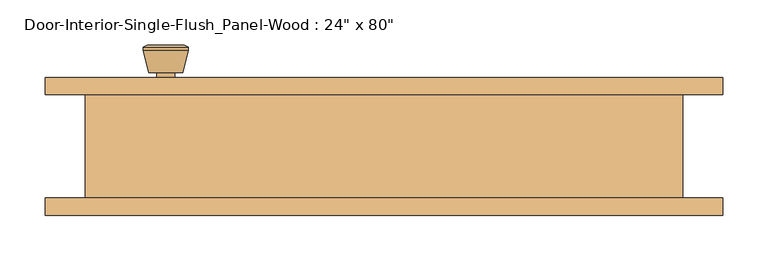
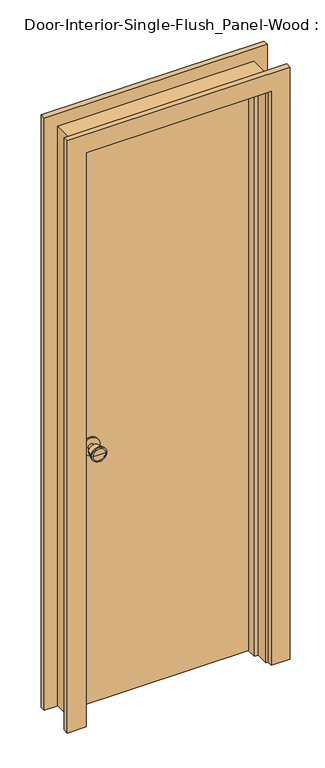
"""IFC4 building model written with IfcOpenShell, lengths in millimetres: door geometry."""

from ifc_helpers import new_model, si_unit, point, frame, frame_2d, origin, origin_with_axes, place, context, project, spatial, polyline, circle_curve, trimmed, segment, composite_curve, outline, extrude, faceted_brep, source, transform, mapped, element, save
from ifc_brep_helpers import plane_surface, cylinder_surface, revolved_surface, advanced_brep


def door_0e119d28(model_context):
    return source(origin(), model_context, "Body", "SolidModel", [
        advanced_brep(
        [(-241.3, 13.05, 914.4), (-231.3, 13.05, 914.4), (-251.3, 13.05, 914.4), (-220.8241324, -35.95, 914.4), (-241.3, -35.95, 914.4), (-261.7758676, -35.95, 914.4), (-216.3, -34.1221319, 914.4), (-266.3, -34.1221319, 914.4), (-216.3, -30.6584537, 914.4), (-266.3, -30.6584537, 914.4), (-222.663764, -5.95, 914.4), (-259.936236, -5.95, 914.4), (-231.3, -5.95, 914.4), (-251.3, -5.95, 914.4)],
        [
            (0, 1),
            (1, 2, circle_curve(frame((-241.3, 13.05, 914.4), z_axis=(0.0, 1.0, 0.0), x_axis=(-1.0, 0.0, 0.0)), 10.0)),
            (2, 0),
            (2, 1, circle_curve(frame((-241.3, 13.05, 914.4), z_axis=(0.0, 1.0, 0.0), x_axis=(-1.0, 0.0, 0.0)), 10.0)),
            (3, 4),
            (4, 5),
            (5, 3, circle_curve(frame((-241.3, -35.95, 914.4), z_axis=(0.0, -1.0, 0.0), x_axis=(-1.0, 0.0, 0.0)), 20.4758676)),
            (3, 5, circle_curve(frame((-241.3, -35.95, 914.4), z_axis=(0.0, -1.0, 0.0), x_axis=(-1.0, 0.0, 0.0)), 20.4758676)),
            (6, 3),
            (5, 7),
            (7, 6, circle_curve(frame((-241.3, -34.1221319, 914.4), z_axis=(0.0, -1.0, 0.0), x_axis=(-1.0, 0.0, 0.0)), 25.0)),
            (6, 7, circle_curve(frame((-241.3, -34.1221319, 914.4), z_axis=(0.0, -1.0, 0.0), x_axis=(-1.0, 0.0, 0.0)), 25.0)),
            (8, 6),
            (7, 9),
            (9, 8, circle_curve(frame((-241.3, -30.6584537, 914.4), z_axis=(0.0, -1.0, 0.0), x_axis=(-1.0, 0.0, 0.0)), 25.0)),
            (8, 9, circle_curve(frame((-241.3, -30.6584537, 914.4), z_axis=(0.0, -1.0, 0.0), x_axis=(-1.0, 0.0, 0.0)), 25.0)),
            (10, 8),
            (9, 11),
            (11, 10, circle_curve(frame((-241.3, -5.95, 914.4), z_axis=(0.0, -1.0, 0.0), x_axis=(-1.0, 0.0, 0.0)), 18.636236)),
            (10, 11, circle_curve(frame((-241.3, -5.95, 914.4), z_axis=(0.0, -1.0, 0.0), x_axis=(-1.0, 0.0, 0.0)), 18.636236)),
            (12, 10),
            (11, 13),
            (13, 12, circle_curve(frame((-241.3, -5.95, 914.4), z_axis=(0.0, -1.0, 0.0), x_axis=(-1.0, 0.0, 0.0)), 10.0)),
            (12, 13, circle_curve(frame((-241.3, -5.95, 914.4), z_axis=(0.0, -1.0, 0.0), x_axis=(-1.0, 0.0, 0.0)), 10.0)),
            (1, 12),
            (13, 2),
        ],
        [
            plane_surface(frame((-241.3, 13.05, 914.4), z_axis=(0.0, 1.0, 0.0), x_axis=(-1.0, 0.0, 0.0))),
            plane_surface(frame((-241.3, -35.95, 914.4), z_axis=(0.0, -1.0, 0.0), x_axis=(-1.0, 0.0, 0.0))),
            revolved_surface(polyline([(-261.7758676, -35.95, 914.4), (-266.3, -34.1221319, 914.4)]), (-241.3, 13.05, 914.4), (0.0, 1.0, 0.0)),
            cylinder_surface(frame((-241.3, 13.05, 914.4), z_axis=(0.0, 1.0, 0.0), x_axis=(-1.0, 0.0, 0.0)), 25.0),
            revolved_surface(polyline([(-266.3, -30.6584537, 914.4), (-259.936236, -5.95, 914.4)]), (-241.3, 13.05, 914.4), (0.0, 1.0, 0.0)),
            plane_surface(frame((-241.3, -5.95, 914.4), z_axis=(0.0, 1.0, 0.0), x_axis=(-1.0, 0.0, 0.0))),
            cylinder_surface(frame((-241.3, 13.05, 914.4), z_axis=(0.0, 1.0, 0.0), x_axis=(-1.0, 0.0, 0.0)), 10.0),
        ],
        [
            (0, [[1, 2, 3]]),
            (0, [[-3, 4, -1]]),
            (1, [[5, 6, 7]]),
            (1, [[-6, -5, 8]]),
            (2, [[9, -7, 10, 11]]),
            (2, [[-10, -8, -9, 12]]),
            (3, [[13, -11, 14, 15]]),
            (3, [[-14, -12, -13, 16]]),
            (4, [[17, -15, 18, 19]]),
            (4, [[-18, -16, -17, 20]]),
            (5, [[21, -19, 22, 23]]),
            (5, [[-22, -20, -21, 24]]),
            (6, [[25, -23, 26, -2]]),
            (6, [[-26, -24, -25, -4]]),
        ],
    ),
        extrude(outline(composite_curve([segment(trimmed(circle_curve(frame_2d((914.4, -241.3)), 30.0), [point((914.4, -271.3))], [point((914.4, -211.3))], False, "CARTESIAN"), True, "CONTINUOUS"), segment(trimmed(circle_curve(frame_2d((914.4, -241.3)), 30.0), [point((914.4, -211.3))], [point((914.4, -271.3))], False, "CARTESIAN"), True, "CONTINUOUS")], self_intersect=False)), frame((0.0, 13.05, 0.0), z_axis=(0.0, 1.0, 0.0), x_axis=(0.0, 0.0, 1.0)), (0.0, 0.0, 1.0), 6.0),
        advanced_brep(
        [(-241.3, 59.975, 914.4), (-251.3, 59.975, 914.4), (-231.3, 59.975, 914.4), (-220.8241324, 108.975, 914.4), (-261.7758676, 108.975, 914.4), (-241.3, 108.975, 914.4), (-216.3, 107.1471319, 914.4), (-266.3, 107.1471319, 914.4), (-216.3, 103.6834537, 914.4), (-266.3, 103.6834537, 914.4), (-222.663764, 78.975, 914.4), (-259.936236, 78.975, 914.4), (-231.3, 78.975, 914.4), (-251.3, 78.975, 914.4)],
        [
            (0, 1),
            (1, 2, circle_curve(frame((-241.3, 59.975, 914.4), z_axis=(0.0, -1.0, 0.0), x_axis=(-1.0, 0.0, 0.0)), 10.0)),
            (2, 0),
            (2, 1, circle_curve(frame((-241.3, 59.975, 914.4), z_axis=(0.0, -1.0, 0.0), x_axis=(-1.0, 0.0, 0.0)), 10.0)),
            (3, 4, circle_curve(frame((-241.3, 108.975, 914.4), z_axis=(0.0, 1.0, 0.0), x_axis=(-1.0, 0.0, 0.0)), 20.4758676)),
            (4, 5),
            (5, 3),
            (4, 3, circle_curve(frame((-241.3, 108.975, 914.4), z_axis=(0.0, 1.0, 0.0), x_axis=(-1.0, 0.0, 0.0)), 20.4758676)),
            (6, 7, circle_curve(frame((-241.3, 107.1471319, 914.4), z_axis=(0.0, 1.0, 0.0), x_axis=(-1.0, 0.0, 0.0)), 25.0)),
            (7, 4),
            (3, 6),
            (7, 6, circle_curve(frame((-241.3, 107.1471319, 914.4), z_axis=(0.0, 1.0, 0.0), x_axis=(-1.0, 0.0, 0.0)), 25.0)),
            (8, 9, circle_curve(frame((-241.3, 103.6834537, 914.4), z_axis=(0.0, 1.0, 0.0), x_axis=(-1.0, 0.0, 0.0)), 25.0)),
            (9, 7),
            (6, 8),
            (9, 8, circle_curve(frame((-241.3, 103.6834537, 914.4), z_axis=(0.0, 1.0, 0.0), x_axis=(-1.0, 0.0, 0.0)), 25.0)),
            (10, 11, circle_curve(frame((-241.3, 78.975, 914.4), z_axis=(0.0, 1.0, 0.0), x_axis=(-1.0, 0.0, 0.0)), 18.636236)),
            (11, 9),
            (8, 10),
            (11, 10, circle_curve(frame((-241.3, 78.975, 914.4), z_axis=(0.0, 1.0, 0.0), x_axis=(-1.0, 0.0, 0.0)), 18.636236)),
            (12, 13, circle_curve(frame((-241.3, 78.975, 914.4), z_axis=(0.0, 1.0, 0.0), x_axis=(-1.0, 0.0, 0.0)), 10.0)),
            (13, 11),
            (10, 12),
            (13, 12, circle_curve(frame((-241.3, 78.975, 914.4), z_axis=(0.0, 1.0, 0.0), x_axis=(-1.0, 0.0, 0.0)), 10.0)),
            (1, 13),
            (12, 2),
        ],
        [
            plane_surface(frame((-241.3, 59.975, 914.4), z_axis=(0.0, -1.0, 0.0), x_axis=(-1.0, 0.0, 0.0))),
            plane_surface(frame((-241.3, 108.975, 914.4), z_axis=(0.0, 1.0, 0.0), x_axis=(-1.0, 0.0, 0.0))),
            revolved_surface(polyline([(-261.7758676, 108.975, 914.4), (-266.3, 107.1471319, 914.4)]), (-241.3, 59.975, 914.4), (0.0, -1.0, 0.0)),
            cylinder_surface(frame((-241.3, 59.975, 914.4), z_axis=(0.0, -1.0, 0.0), x_axis=(-1.0, 0.0, 0.0)), 25.0),
            revolved_surface(polyline([(-266.3, 103.6834537, 914.4), (-259.936236, 78.975, 914.4)]), (-241.3, 59.975, 914.4), (0.0, -1.0, 0.0)),
            plane_surface(frame((-241.3, 78.975, 914.4), z_axis=(0.0, -1.0, 0.0), x_axis=(-1.0, 0.0, 0.0))),
            cylinder_surface(frame((-241.3, 59.975, 914.4), z_axis=(0.0, -1.0, 0.0), x_axis=(-1.0, 0.0, 0.0)), 10.0),
        ],
        [
            (0, [[1, 2, 3]]),
            (0, [[-3, 4, -1]]),
            (1, [[5, 6, 7]]),
            (1, [[8, -7, -6]]),
            (2, [[9, 10, -5, 11]]),
            (2, [[12, -11, -8, -10]]),
            (3, [[13, 14, -9, 15]]),
            (3, [[16, -15, -12, -14]]),
            (4, [[17, 18, -13, 19]]),
            (4, [[20, -19, -16, -18]]),
            (5, [[21, 22, -17, 23]]),
            (5, [[24, -23, -20, -22]]),
            (6, [[-2, 25, -21, 26]]),
            (6, [[-4, -26, -24, -25]]),
        ],
    ),
        extrude(outline(composite_curve([segment(trimmed(circle_curve(frame_2d((914.4, -241.3)), 30.0), [point((914.4, -271.3))], [point((914.4, -211.3))], False, "CARTESIAN"), True, "CONTINUOUS"), segment(trimmed(circle_curve(frame_2d((914.4, -241.3)), 30.0), [point((914.4, -211.3))], [point((914.4, -271.3))], False, "CARTESIAN"), True, "CONTINUOUS")], self_intersect=False)), frame((0.0, 53.975, 0.0), z_axis=(0.0, 1.0, 0.0), x_axis=(0.0, 0.0, 1.0)), (0.0, 0.0, 1.0), 6.0),
        faceted_brep([(330.2, 53.975, 0.0), (330.2, -60.325, 0.0), (304.8, -60.325, 0.0), (304.8, -15.875, 0.0), (292.1, -15.875, 0.0), (292.1, 19.05, 0.0), (304.8, 19.05, 0.0), (304.8, 53.975, 0.0), (330.2, 53.975, 2057.4), (330.2, -60.325, 2057.4), (-330.2, -60.325, 2057.4), (-330.2, -60.325, 0.0), (-304.8, -60.325, 0.0), (-304.8, -60.325, 2032.0), (304.8, -60.325, 2032.0), (304.8, -15.875, 2032.0), (-304.8, -15.875, 2032.0), (-304.8, -15.875, 0.0), (-292.1, -15.875, 0.0), (-292.1, -15.875, 2019.3), (292.1, -15.875, 2019.3), (292.1, 19.05, 2019.3), (-292.1, 19.05, 2019.3), (-292.1, 19.05, 0.0), (-304.8, 19.05, 0.0), (-304.8, 19.05, 2032.0), (304.8, 19.05, 2032.0), (304.8, 53.975, 2032.0), (-304.8, 53.975, 2032.0), (-304.8, 53.975, 0.0), (-330.2, 53.975, 0.0), (-330.2, 53.975, 2057.4)], [[[0, 1, 2, 3, 4, 5, 6, 7]], [[1, 0, 8, 9]], [[2, 1, 9, 10, 11, 12, 13, 14]], [[3, 2, 14, 15]], [[4, 3, 15, 16, 17, 18, 19, 20]], [[5, 4, 20, 21]], [[6, 5, 21, 22, 23, 24, 25, 26]], [[7, 6, 26, 27]], [[0, 7, 27, 28, 29, 30, 31, 8]], [[9, 8, 31, 10]], [[15, 14, 13, 16]], [[21, 20, 19, 22]], [[27, 26, 25, 28]], [[30, 29, 24, 23, 18, 17, 12, 11]], [[10, 31, 30, 11]], [[16, 13, 12, 17]], [[22, 19, 18, 23]], [[28, 25, 24, 29]]]),
        extrude(outline(polyline([(304.8, 19.05), (-304.8, 19.05), (-304.8, 53.975), (304.8, 53.975), (304.8, 19.05)])), origin_with_axes(), (0.0, 0.0, 1.0), 2032.0),
        extrude(outline(polyline([(0.0, 311.15), (0.0, 374.65), (2101.85, 374.65), (2101.85, -374.65), (0.0, -374.65), (0.0, -311.15), (2038.35, -311.15), (2038.35, 311.15), (0.0, 311.15)])), frame((0.0, 53.975, 0.0), z_axis=(0.0, 1.0, 0.0), x_axis=(0.0, 0.0, 1.0)), (0.0, 0.0, 1.0), 19.05),
        extrude(outline(polyline([(0.0, 311.15), (0.0, 374.65), (2101.85, 374.65), (2101.85, -374.65), (0.0, -374.65), (0.0, -311.15), (2038.35, -311.15), (2038.35, 311.15), (0.0, 311.15)])), frame((0.0, -79.375, 0.0), z_axis=(0.0, 1.0, 0.0), x_axis=(0.0, 0.0, 1.0)), (0.0, 0.0, 1.0), 19.05),
    ])


if __name__ == "__main__":
    model = new_model("IFC4")
    model_context = context("Model", 3, world=origin())
    ifc_project = project(units=[si_unit("LENGTHUNIT", "METRE", prefix="MILLI")], contexts=[model_context])
    site = spatial("IfcSite", under=ifc_project)
    building = spatial("IfcBuilding", under=site)
    placement = place(None, origin())
    door_shape = door_0e119d28(model_context)
    element("IfcDoor", 1, ObjectType="Door-Interior-Single-Flush_Panel-Wood : 24\" x 80\"", at=placement, inside=building, context=model_context, shape_type="MappedRepresentation", body=[
        mapped(door_shape, transform((0.0, 0.0, 0.0), x_axis=(1.0, 0.0, 0.0), y_axis=(0.0, 1.0, 0.0), z_axis=(0.0, 0.0, 1.0))),
    ])
    save(model, "model.ifc")

# Revit data of these elements
# Type "Door-Interior-Single-Flush_Panel-Wood : 24\" x 80\""
#   Type Mark = "12"
#   Assembly Code = "C1020300"
#   Analytic Construction = "Wooden"
#   Thickness = 0' - 1 3/8"
#   Thermal Resistance (R) = 2.5876 (h·ft²·°F)/BTU
#   Swing Angle [instance default] = 90.00°
#   Rough Width = 2' - 2"
#   Rough Height = 6' - 9"
#   Height = 6' - 8"
#   Width = 2' - 0"
#   Heat Transfer Coefficient (U) = 0.3865 BTU/(h·ft²·°F)
#   Trim Material = Cherry
#   Panel Material = Cherry
#   Frame Material = Cherry
#   Door Handle Material = Aluminum
#   Visual Light Transmittance = 0
#   Solar Heat Gain Coefficient = 0
#   Wall Closure = (empty or 0)
#   Function = (empty or 0)
# Element 1 (IfcDoor, "Door-Interior-Single-Flush_Panel-Wood : 24\" x 80\"")
#   Materials on its faces: "Cherry", "Aluminum"
# Materials
#   "Cherry": class "Wood", colour RGB 226 177 128, transparency 0, Description = "Prunus Serotina", Cost = 0
#   "Aluminum": class "Metal", colour RGB 247 247 247, transparency 0, Description = "Aluminum 6061", Cost = 0
